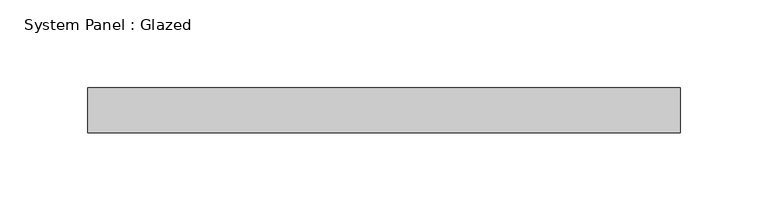
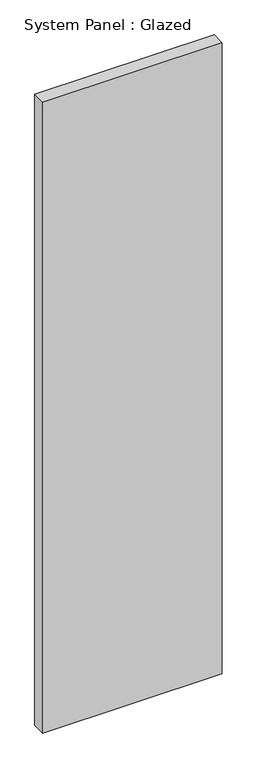
"""IFC4 building model written with IfcOpenShell, lengths in millimetres: plate geometry, System Panel : Glazed."""

from ifc_helpers import new_model, si_unit, origin, origin_with_axes, place, context, project, spatial, polyline, outline, extrude, source, transform, mapped, element, save


def system_panel_glazed_ce423334(model_context):
    return source(origin(), model_context, "Body", "SweptSolid", [
        extrude(outline(polyline([(168.275, 19.05), (-168.275, 19.05), (-168.275, 44.45), (168.275, 44.45), (168.275, 19.05)])), origin_with_axes(), (0.0, 0.0, 1.0), 1249.6336497),
    ])


if __name__ == "__main__":
    model = new_model("IFC4")
    model_context = context("Model", 3, world=origin())
    ifc_project = project(units=[si_unit("LENGTHUNIT", "METRE", prefix="MILLI")], contexts=[model_context])
    site = spatial("IfcSite", under=ifc_project)
    building = spatial("IfcBuilding", under=site)
    placement = place(None, origin())
    system_panel_glazed_shape = system_panel_glazed_ce423334(model_context)
    element("IfcPlate", 1, ObjectType="System Panel : Glazed", at=placement, inside=building, context=model_context, shape_type="MappedRepresentation", body=[
        mapped(system_panel_glazed_shape, transform((0.0, 0.0, 0.0), x_axis=(1.0, 0.0, 0.0), y_axis=(0.0, 1.0, 0.0), z_axis=(0.0, 0.0, 1.0))),
    ])
    save(model, "model.ifc")

# Revit data of these elements
# Type "System Panel : Glazed"
#   Construction Type Id = "GSP4R"
#   Analytic Construction = "1/8 in Pilkington single glazing"
#   Visual Light Transmittance = 0.9
#   Solar Heat Gain Coefficient = 0.86
#   Heat Transfer Coefficient (U) = 1.18115 BTU/(h·ft²·°F)
#   Define Thermal Properties by = 1
# Element 1 (IfcPlate, "System Panel : Glazed")
#   Materials on its faces: "Glass"
# Materials
#   "Glass": class "Glass", colour RGB 0 128 192, transparency 0.75, Description = "Soda Lime Glass", Cost = 0
